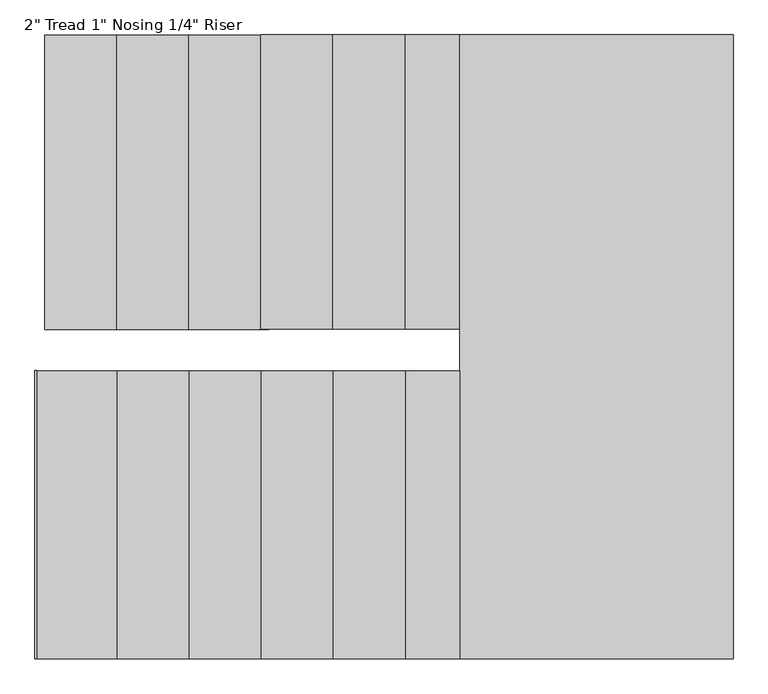
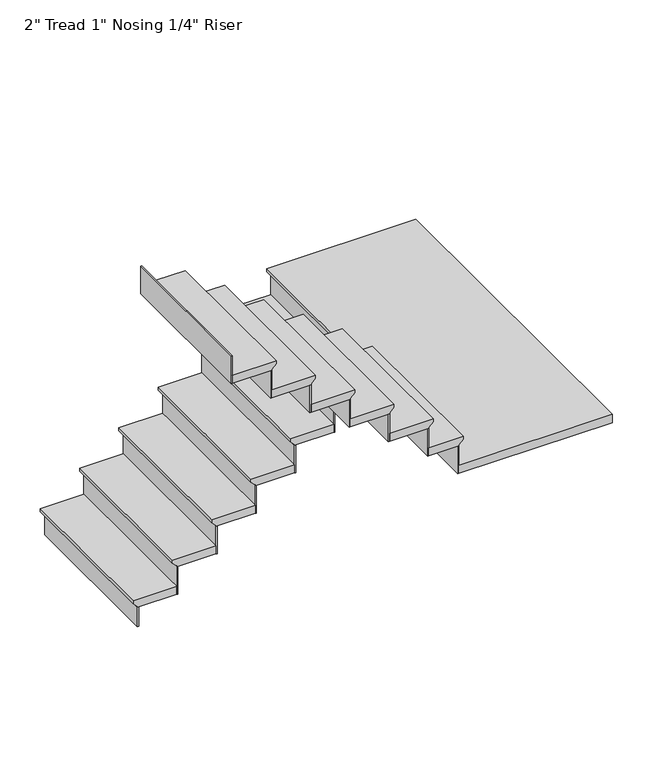
"""IFC4 building model written with IfcOpenShell, lengths in millimetres: stair flight geometry."""

from ifc_helpers import new_model, si_unit, origin, place, context, project, spatial, faceted_brep, source, transform, mapped, element, save


def stair_flight_6f98f22d(model_context):
    return source(origin(), model_context, "Body", "Brep", [
        faceted_brep([(-1022.6415352, -3861.2539367, 6551.0833333), (-1022.6415352, -3861.2539367, 6570.1333333), (-1022.6415352, -2926.4769687, 6570.1333333), (-1022.6415352, -2926.4769687, 6551.0833333), (-997.2415352, -3861.2539367, 6525.6833333), (-997.2415352, -2926.4769687, 6525.6833333), (-768.6415352, -3861.2539367, 6570.1333333), (-768.6415352, -2926.4769687, 6570.1333333), (-997.2415352, -2926.4769687, 6519.3333333), (-768.6415352, -2926.4769687, 6519.3333333), (-768.6415352, -3861.2539367, 6519.3333333), (-997.2415352, -3861.2539367, 6519.3333333)], [[[0, 1, 2, 3]], [[4, 0, 3, 5]], [[2, 1, 6, 7]], [[8, 9, 10, 11]], [[2, 7, 9, 8, 5, 3]], [[8, 11, 4, 5]], [[6, 1, 0, 4, 11, 10]], [[7, 6, 10, 9]]]),
        faceted_brep([(-997.2415352, -3861.2539367, 6519.3333333), (-997.2415352, -3861.2539367, 6400.8), (-990.8915352, -3861.2539367, 6400.8), (-990.8915352, -3861.2539367, 6519.3333333), (-997.2415352, -2926.4769687, 6519.3333333), (-990.8915352, -2926.4769687, 6519.3333333), (-990.8915352, -2926.4769687, 6400.8), (-997.2415352, -2926.4769687, 6400.8)], [[[0, 1, 2, 3]], [[4, 5, 6, 7]], [[1, 0, 4, 7]], [[2, 1, 7, 6]], [[3, 2, 6, 5]], [[0, 3, 5, 4]]]),
        faceted_brep([(-768.6415352, -3861.2539367, 6688.6666667), (-768.6415352, -3861.2539367, 6519.3333333), (-762.2915352, -3861.2539367, 6519.3333333), (-762.2915352, -3861.2539367, 6688.6666667), (-768.6415352, -2926.4769687, 6688.6666667), (-762.2915352, -2926.4769687, 6688.6666667), (-762.2915352, -2926.4769687, 6519.3333333), (-768.6415352, -2926.4769687, 6519.3333333)], [[[0, 1, 2, 3]], [[4, 5, 6, 7]], [[1, 0, 4, 7]], [[2, 1, 7, 6]], [[3, 2, 6, 5]], [[0, 3, 5, 4]]]),
        faceted_brep([(-794.0415352, -2926.4769687, 6739.4666667), (-794.0415352, -3861.2539367, 6739.4666667), (-540.0415352, -3861.2539367, 6739.4666667), (-540.0415352, -2926.4769687, 6739.4666667), (-768.6415352, -2926.4769687, 6688.6666667), (-540.0415352, -2926.4769687, 6688.6666667), (-540.0415352, -3861.2539367, 6688.6666667), (-768.6415352, -3861.2539367, 6688.6666667), (-768.6415352, -2926.4769687, 6695.0166667), (-794.0415352, -2926.4769687, 6720.4166667), (-768.6415352, -3861.2539367, 6695.0166667), (-794.0415352, -3861.2539367, 6720.4166667)], [[[0, 1, 2, 3]], [[4, 5, 6, 7]], [[0, 3, 5, 4, 8, 9]], [[4, 7, 10, 8]], [[2, 1, 11, 10, 7, 6]], [[3, 2, 6, 5]], [[11, 1, 0, 9]], [[10, 11, 9, 8]]]),
        faceted_brep([(-540.0415352, -3861.2539367, 6858.0), (-540.0415352, -3861.2539367, 6688.6666667), (-533.6915352, -3861.2539367, 6688.6666667), (-533.6915352, -3861.2539367, 6858.0), (-540.0415352, -2926.4769687, 6858.0), (-533.6915352, -2926.4769687, 6858.0), (-533.6915352, -2926.4769687, 6688.6666667), (-540.0415352, -2926.4769687, 6688.6666667)], [[[0, 1, 2, 3]], [[4, 5, 6, 7]], [[1, 0, 4, 7]], [[2, 1, 7, 6]], [[3, 2, 6, 5]], [[0, 3, 5, 4]]]),
        faceted_brep([(-565.4415352, -2926.4769687, 6908.8), (-565.4415352, -3861.2539367, 6908.8), (-311.4415352, -3861.2539367, 6908.8), (-311.4415352, -2926.4769687, 6908.8), (-540.0415352, -2926.4769687, 6858.0), (-311.4415352, -2926.4769687, 6858.0), (-311.4415352, -3861.2539367, 6858.0), (-540.0415352, -3861.2539367, 6858.0), (-540.0415352, -2926.4769687, 6864.35), (-565.4415352, -2926.4769687, 6889.75), (-540.0415352, -3861.2539367, 6864.35), (-565.4415352, -3861.2539367, 6889.75)], [[[0, 1, 2, 3]], [[4, 5, 6, 7]], [[0, 3, 5, 4, 8, 9]], [[4, 7, 10, 8]], [[2, 1, 11, 10, 7, 6]], [[3, 2, 6, 5]], [[11, 1, 0, 9]], [[10, 11, 9, 8]]]),
        faceted_brep([(-311.4415352, -3861.2539367, 7027.3333333), (-311.4415352, -3861.2539367, 6858.0), (-305.0915352, -3861.2539367, 6858.0), (-305.0915352, -3861.2539367, 7027.3333333), (-311.4415352, -2926.4769687, 7027.3333333), (-305.0915352, -2926.4769687, 7027.3333333), (-305.0915352, -2926.4769687, 6858.0), (-311.4415352, -2926.4769687, 6858.0)], [[[0, 1, 2, 3]], [[4, 5, 6, 7]], [[1, 0, 4, 7]], [[2, 1, 7, 6]], [[3, 2, 6, 5]], [[0, 3, 5, 4]]]),
        faceted_brep([(-336.8415352, -2926.4769687, 7078.1333333), (-336.8415352, -3861.2539367, 7078.1333333), (-82.8415352, -3861.2539367, 7078.1333333), (-82.8415352, -2926.4769687, 7078.1333333), (-311.4415352, -2926.4769687, 7027.3333333), (-82.8415352, -2926.4769687, 7027.3333333), (-82.8415352, -3861.2539367, 7027.3333333), (-311.4415352, -3861.2539367, 7027.3333333), (-311.4415352, -2926.4769687, 7033.6833333), (-336.8415352, -2926.4769687, 7059.0833333), (-311.4415352, -3861.2539367, 7033.6833333), (-336.8415352, -3861.2539367, 7059.0833333)], [[[0, 1, 2, 3]], [[4, 5, 6, 7]], [[0, 3, 5, 4, 8, 9]], [[4, 7, 10, 8]], [[2, 1, 11, 10, 7, 6]], [[3, 2, 6, 5]], [[11, 1, 0, 9]], [[10, 11, 9, 8]]]),
        faceted_brep([(-82.8415352, -3861.2539367, 7196.6666667), (-82.8415352, -3861.2539367, 7027.3333333), (-76.4915352, -3861.2539367, 7027.3333333), (-76.4915352, -3861.2539367, 7196.6666667), (-82.8415352, -2926.4769687, 7196.6666667), (-76.4915352, -2926.4769687, 7196.6666667), (-76.4915352, -2926.4769687, 7027.3333333), (-82.8415352, -2926.4769687, 7027.3333333)], [[[0, 1, 2, 3]], [[4, 5, 6, 7]], [[1, 0, 4, 7]], [[2, 1, 7, 6]], [[3, 2, 6, 5]], [[0, 3, 5, 4]]]),
        faceted_brep([(-108.2415352, -2926.4769687, 7247.4666667), (-108.2415352, -3861.2539367, 7247.4666667), (145.7584648, -3861.2539367, 7247.4666667), (145.7584648, -2926.4769687, 7247.4666667), (-82.8415352, -2926.4769687, 7196.6666667), (145.7584648, -2926.4769687, 7196.6666667), (145.7584648, -3861.2539367, 7196.6666667), (-82.8415352, -3861.2539367, 7196.6666667), (-82.8415352, -2926.4769687, 7203.0166667), (-108.2415352, -2926.4769687, 7228.4166667), (-82.8415352, -3861.2539367, 7203.0166667), (-108.2415352, -3861.2539367, 7228.4166667)], [[[0, 1, 2, 3]], [[4, 5, 6, 7]], [[0, 3, 5, 4, 8, 9]], [[4, 7, 10, 8]], [[2, 1, 11, 10, 7, 6]], [[3, 2, 6, 5]], [[11, 1, 0, 9]], [[10, 11, 9, 8]]]),
        faceted_brep([(145.7584648, -3861.2539367, 7366.0), (145.7584648, -3861.2539367, 7196.6666667), (152.1084648, -3861.2539367, 7196.6666667), (152.1084648, -3861.2539367, 7366.0), (145.7584648, -2926.4769687, 7366.0), (152.1084648, -2926.4769687, 7366.0), (152.1084648, -2926.4769687, 7196.6666667), (145.7584648, -2926.4769687, 7196.6666667)], [[[0, 1, 2, 3]], [[4, 5, 6, 7]], [[1, 0, 4, 7]], [[2, 1, 7, 6]], [[3, 2, 6, 5]], [[0, 3, 5, 4]]]),
        faceted_brep([(120.3584648, -2926.4769687, 7416.8), (120.3584648, -3861.2539367, 7416.8), (320.0221038, -3861.2539367, 7416.8), (320.0221038, -2926.4769687, 7416.8), (145.7584648, -2926.4769687, 7366.0), (320.0221038, -2926.4769687, 7366.0), (320.0221038, -3861.2539367, 7366.0), (145.7584648, -3861.2539367, 7366.0), (145.7584648, -2926.4769687, 7372.35), (120.3584648, -2926.4769687, 7397.75), (145.7584648, -3861.2539367, 7372.35), (120.3584648, -3861.2539367, 7397.75)], [[[0, 1, 2, 3]], [[4, 5, 6, 7]], [[0, 3, 5, 4, 8, 9]], [[4, 7, 10, 8]], [[2, 1, 11, 10, 7, 6]], [[3, 2, 6, 5]], [[11, 1, 0, 9]], [[10, 11, 9, 8]]]),
        faceted_brep([(320.0221038, -3861.2539367, 7535.3333333), (320.0221038, -3861.2539367, 7366.0), (326.3721038, -3861.2539367, 7366.0), (326.3721038, -3861.2539367, 7535.3333333), (320.0221038, -2926.4769687, 7535.3333333), (326.3721038, -2926.4769687, 7535.3333333), (326.3721038, -2926.4769687, 7366.0), (320.0221038, -2926.4769687, 7366.0)], [[[0, 1, 2, 3]], [[4, 5, 6, 7]], [[1, 0, 4, 7]], [[2, 1, 7, 6]], [[3, 2, 6, 5]], [[0, 3, 5, 4]]]),
        faceted_brep([(269.2221038, -4907.6769687, 7586.1333333), (1161.7584648, -4907.6769687, 7586.1333333), (1161.7584648, -2926.4769687, 7586.1333333), (294.6221038, -2926.4769687, 7586.1333333), (294.6221038, -3993.2769687, 7586.1333333), (269.2221038, -3993.2769687, 7586.1333333), (1161.7584648, -4907.6769687, 7535.3333333), (269.2221038, -4907.6769687, 7535.3333333), (269.2221038, -3993.2769687, 7535.3333333), (294.6221038, -3993.2769687, 7535.3333333), (294.6221038, -3861.2539367, 7535.3333333), (320.0221038, -3861.2539367, 7535.3333333), (320.0221038, -2926.4769687, 7535.3333333), (1161.7584648, -2926.4769687, 7535.3333333), (320.0221038, -2926.4769687, 7541.6833333), (294.6221038, -2926.4769687, 7567.0833333), (320.0221038, -3861.2539367, 7541.6833333), (294.6221038, -3861.2539367, 7567.0833333)], [[[0, 1, 2, 3, 4, 5]], [[6, 7, 8, 9, 10, 11, 12, 13]], [[1, 0, 7, 6]], [[2, 1, 6, 13]], [[3, 2, 13, 12, 14, 15]], [[12, 11, 16, 14]], [[11, 10, 17, 16]], [[4, 3, 15, 17, 10, 9]], [[5, 4, 9, 8]], [[0, 5, 8, 7]], [[15, 14, 16, 17]]]),
        faceted_brep([(269.2221038, -3993.2769687, 7704.6666667), (269.2221038, -3993.2769687, 7535.3333333), (262.8721038, -3993.2769687, 7535.3333333), (262.8721038, -3993.2769687, 7704.6666667), (269.2221038, -4907.6769687, 7704.6666667), (262.8721038, -4907.6769687, 7704.6666667), (262.8721038, -4907.6769687, 7535.3333333), (269.2221038, -4907.6769687, 7535.3333333)], [[[0, 1, 2, 3]], [[4, 5, 6, 7]], [[1, 0, 4, 7]], [[2, 1, 7, 6]], [[3, 2, 6, 5]], [[0, 3, 5, 4]]]),
        faceted_brep([(294.6221038, -4907.6769687, 7755.4666667), (294.6221038, -3993.2769687, 7755.4666667), (94.9584648, -3993.2769687, 7755.4666667), (94.9584648, -4907.6769687, 7755.4666667), (269.2221038, -4907.6769687, 7704.6666667), (94.9584648, -4907.6769687, 7704.6666667), (94.9584648, -3993.2769687, 7704.6666667), (269.2221038, -3993.2769687, 7704.6666667), (269.2221038, -4907.6769687, 7711.0166667), (294.6221038, -4907.6769687, 7736.4166667), (269.2221038, -3993.2769687, 7711.0166667), (294.6221038, -3993.2769687, 7736.4166667)], [[[0, 1, 2, 3]], [[4, 5, 6, 7]], [[0, 3, 5, 4, 8, 9]], [[4, 7, 10, 8]], [[2, 1, 11, 10, 7, 6]], [[3, 2, 6, 5]], [[11, 1, 0, 9]], [[10, 11, 9, 8]]]),
        faceted_brep([(94.9584648, -3993.2769687, 7874.0), (94.9584648, -3993.2769687, 7704.6666667), (88.6084648, -3993.2769687, 7704.6666667), (88.6084648, -3993.2769687, 7874.0), (94.9584648, -4907.6769687, 7874.0), (88.6084648, -4907.6769687, 7874.0), (88.6084648, -4907.6769687, 7704.6666667), (94.9584648, -4907.6769687, 7704.6666667)], [[[0, 1, 2, 3]], [[4, 5, 6, 7]], [[1, 0, 4, 7]], [[2, 1, 7, 6]], [[3, 2, 6, 5]], [[0, 3, 5, 4]]]),
        faceted_brep([(120.3584648, -4907.6769687, 7924.8), (120.3584648, -3993.2769687, 7924.8), (-133.6415352, -3993.2769687, 7924.8), (-133.6415352, -4907.6769687, 7924.8), (94.9584648, -4907.6769687, 7874.0), (-133.6415352, -4907.6769687, 7874.0), (-133.6415352, -3993.2769687, 7874.0), (94.9584648, -3993.2769687, 7874.0), (94.9584648, -4907.6769687, 7880.35), (120.3584648, -4907.6769687, 7905.75), (94.9584648, -3993.2769687, 7880.35), (120.3584648, -3993.2769687, 7905.75)], [[[0, 1, 2, 3]], [[4, 5, 6, 7]], [[0, 3, 5, 4, 8, 9]], [[4, 7, 10, 8]], [[2, 1, 11, 10, 7, 6]], [[3, 2, 6, 5]], [[11, 1, 0, 9]], [[10, 11, 9, 8]]]),
        faceted_brep([(-133.6415352, -3993.2769687, 8043.3333333), (-133.6415352, -3993.2769687, 7874.0), (-139.9915352, -3993.2769687, 7874.0), (-139.9915352, -3993.2769687, 8043.3333333), (-133.6415352, -4907.6769687, 8043.3333333), (-139.9915352, -4907.6769687, 8043.3333333), (-139.9915352, -4907.6769687, 7874.0), (-133.6415352, -4907.6769687, 7874.0)], [[[0, 1, 2, 3]], [[4, 5, 6, 7]], [[1, 0, 4, 7]], [[2, 1, 7, 6]], [[3, 2, 6, 5]], [[0, 3, 5, 4]]]),
        faceted_brep([(-108.2415352, -4907.6769687, 8094.1333333), (-108.2415352, -3993.2769687, 8094.1333333), (-362.2415352, -3993.2769687, 8094.1333333), (-362.2415352, -4907.6769687, 8094.1333333), (-133.6415352, -4907.6769687, 8043.3333333), (-362.2415352, -4907.6769687, 8043.3333333), (-362.2415352, -3993.2769687, 8043.3333333), (-133.6415352, -3993.2769687, 8043.3333333), (-133.6415352, -4907.6769687, 8049.6833333), (-108.2415352, -4907.6769687, 8075.0833333), (-133.6415352, -3993.2769687, 8049.6833333), (-108.2415352, -3993.2769687, 8075.0833333)], [[[0, 1, 2, 3]], [[4, 5, 6, 7]], [[0, 3, 5, 4, 8, 9]], [[4, 7, 10, 8]], [[2, 1, 11, 10, 7, 6]], [[3, 2, 6, 5]], [[11, 1, 0, 9]], [[10, 11, 9, 8]]]),
        faceted_brep([(-362.2415352, -3993.2769687, 8212.6666667), (-362.2415352, -3993.2769687, 8043.3333333), (-368.5915352, -3993.2769687, 8043.3333333), (-368.5915352, -3993.2769687, 8212.6666667), (-362.2415352, -4907.6769687, 8212.6666667), (-368.5915352, -4907.6769687, 8212.6666667), (-368.5915352, -4907.6769687, 8043.3333333), (-362.2415352, -4907.6769687, 8043.3333333)], [[[0, 1, 2, 3]], [[4, 5, 6, 7]], [[1, 0, 4, 7]], [[2, 1, 7, 6]], [[3, 2, 6, 5]], [[0, 3, 5, 4]]]),
        faceted_brep([(-336.8415352, -4907.6769687, 8263.4666667), (-336.8415352, -3993.2769687, 8263.4666667), (-590.8415352, -3993.2769687, 8263.4666667), (-590.8415352, -4907.6769687, 8263.4666667), (-362.2415352, -4907.6769687, 8212.6666667), (-590.8415352, -4907.6769687, 8212.6666667), (-590.8415352, -3993.2769687, 8212.6666667), (-362.2415352, -3993.2769687, 8212.6666667), (-362.2415352, -4907.6769687, 8219.0166667), (-336.8415352, -4907.6769687, 8244.4166667), (-362.2415352, -3993.2769687, 8219.0166667), (-336.8415352, -3993.2769687, 8244.4166667)], [[[0, 1, 2, 3]], [[4, 5, 6, 7]], [[0, 3, 5, 4, 8, 9]], [[4, 7, 10, 8]], [[2, 1, 11, 10, 7, 6]], [[3, 2, 6, 5]], [[11, 1, 0, 9]], [[10, 11, 9, 8]]]),
        faceted_brep([(-590.8415352, -3993.2769687, 8382.0), (-590.8415352, -3993.2769687, 8212.6666667), (-597.1915352, -3993.2769687, 8212.6666667), (-597.1915352, -3993.2769687, 8382.0), (-590.8415352, -4907.6769687, 8382.0), (-597.1915352, -4907.6769687, 8382.0), (-597.1915352, -4907.6769687, 8212.6666667), (-590.8415352, -4907.6769687, 8212.6666667)], [[[0, 1, 2, 3]], [[4, 5, 6, 7]], [[1, 0, 4, 7]], [[2, 1, 7, 6]], [[3, 2, 6, 5]], [[0, 3, 5, 4]]]),
        faceted_brep([(-565.4415352, -4907.6769687, 8432.8), (-565.4415352, -3993.2769687, 8432.8), (-819.4415352, -3993.2769687, 8432.8), (-819.4415352, -4907.6769687, 8432.8), (-590.8415352, -4907.6769687, 8382.0), (-819.4415352, -4907.6769687, 8382.0), (-819.4415352, -3993.2769687, 8382.0), (-590.8415352, -3993.2769687, 8382.0), (-590.8415352, -4907.6769687, 8388.35), (-565.4415352, -4907.6769687, 8413.75), (-590.8415352, -3993.2769687, 8388.35), (-565.4415352, -3993.2769687, 8413.75)], [[[0, 1, 2, 3]], [[4, 5, 6, 7]], [[0, 3, 5, 4, 8, 9]], [[4, 7, 10, 8]], [[2, 1, 11, 10, 7, 6]], [[3, 2, 6, 5]], [[11, 1, 0, 9]], [[10, 11, 9, 8]]]),
        faceted_brep([(-819.4415352, -3993.2769687, 8551.3333333), (-819.4415352, -3993.2769687, 8382.0), (-825.7915352, -3993.2769687, 8382.0), (-825.7915352, -3993.2769687, 8551.3333333), (-819.4415352, -4907.6769687, 8551.3333333), (-825.7915352, -4907.6769687, 8551.3333333), (-825.7915352, -4907.6769687, 8382.0), (-819.4415352, -4907.6769687, 8382.0)], [[[0, 1, 2, 3]], [[4, 5, 6, 7]], [[1, 0, 4, 7]], [[2, 1, 7, 6]], [[3, 2, 6, 5]], [[0, 3, 5, 4]]]),
        faceted_brep([(-1048.0415352, -3993.2769687, 8720.6666667), (-1048.0415352, -3993.2769687, 8551.3333333), (-1054.3915352, -3993.2769687, 8551.3333333), (-1054.3915352, -3993.2769687, 8720.6666667), (-1048.0415352, -4907.6769687, 8720.6666667), (-1054.3915352, -4907.6769687, 8720.6666667), (-1054.3915352, -4907.6769687, 8551.3333333), (-1048.0415352, -4907.6769687, 8551.3333333)], [[[0, 1, 2, 3]], [[4, 5, 6, 7]], [[1, 0, 4, 7]], [[2, 1, 7, 6]], [[3, 2, 6, 5]], [[0, 3, 5, 4]]]),
        faceted_brep([(-794.0415352, -4907.6769687, 8602.1333333), (-794.0415352, -3993.2769687, 8602.1333333), (-1048.0415352, -3993.2769687, 8602.1333333), (-1048.0415352, -4907.6769687, 8602.1333333), (-819.4415352, -4907.6769687, 8551.3333333), (-1048.0415352, -4907.6769687, 8551.3333333), (-1048.0415352, -3993.2769687, 8551.3333333), (-819.4415352, -3993.2769687, 8551.3333333), (-819.4415352, -4907.6769687, 8557.6833333), (-794.0415352, -4907.6769687, 8583.0833333), (-819.4415352, -3993.2769687, 8557.6833333), (-794.0415352, -3993.2769687, 8583.0833333)], [[[0, 1, 2, 3]], [[4, 5, 6, 7]], [[0, 3, 5, 4, 8, 9]], [[4, 7, 10, 8]], [[2, 1, 11, 10, 7, 6]], [[3, 2, 6, 5]], [[11, 1, 0, 9]], [[10, 11, 9, 8]]]),
    ])


if __name__ == "__main__":
    model = new_model("IFC4")
    model_context = context("Model", 3, world=origin())
    ifc_project = project(units=[si_unit("LENGTHUNIT", "METRE", prefix="MILLI")], contexts=[model_context])
    site = spatial("IfcSite", under=ifc_project)
    building = spatial("IfcBuilding", under=site)
    placement = place(None, origin())
    stair_flight_shape = stair_flight_6f98f22d(model_context)
    element("IfcStairFlight", 1, ObjectType="2\" Tread 1\" Nosing 1/4\" Riser", at=placement, inside=building, context=model_context, shape_type="MappedRepresentation", body=[
        mapped(stair_flight_shape, transform((0.0, 0.0, 0.0), x_axis=(1.0, 0.0, 0.0), y_axis=(0.0, 1.0, 0.0), z_axis=(0.0, 0.0, 1.0))),
    ])
    save(model, "model.ifc")
